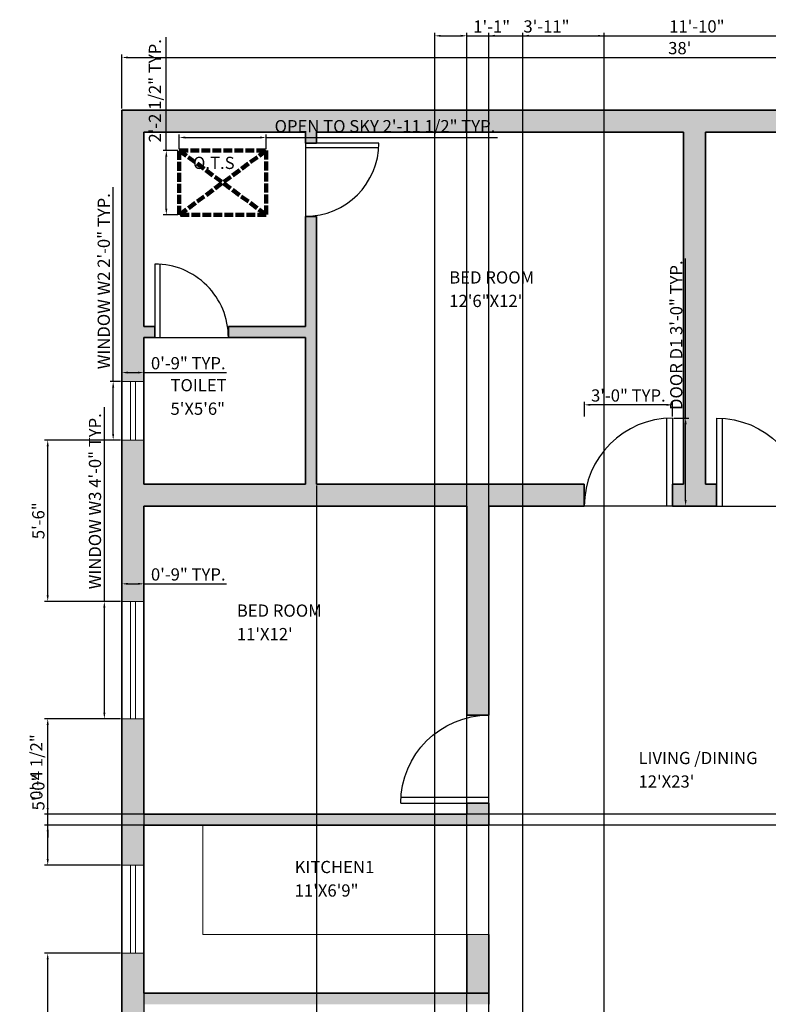
# Model space of a CAD drawing. Units: inches. Extents: x 2263 to 2802, y 2658 to 3310.
# Tile 2 of 3: x 2263 to 2569, y 2902 to 3305. Entities that reach past the tile are written whole.
import ezdxf

# ---------------------------------------------------------------- set-up
doc = ezdxf.new("R2010")
doc.units = ezdxf.units.IN
doc.header["$LTSCALE"] = 0.3
doc.linetypes.add('ACAD_ISO02W100', pattern=[15, 12, -3])
for name, color, linetype, lineweight in [('A-ANNO-DIMS', 2, 'Continuous', 18), ('A-AREA-IDEN', 7, 'Continuous', 18), ('A-DOOR', 3, 'Continuous', 25), ('A-FLOR-FIXT', 8, 'Continuous', 18), ('A-GLAZ', 4, 'Continuous', 18), ('A-ROOF-OVHD', 7, 'ACAD_ISO02W100', 100), ('A-WALL', 7, 'Continuous', 35)]:
    doc.layers.add(name, color=color, linetype=linetype, lineweight=lineweight)
doc.layers.add('A-WALL-PATT', color=18, linetype='Continuous', lineweight=13, true_color=0x000000)
doc.styles.get("Standard").update_dxf_attribs({"font": 'calibri.ttf', "height": 5})
doc.dimstyles.new('ISO-25', dxfattribs={"dimtxt": 5, "dimasz": 2.5, "dimexe": 1.25, "dimexo": 0.625, "dimtad": 1, "dimlunit": 3, "dimtxsty": 'Standard', "dimcen": 2.5, "dimadec": 0, "dimazin": 0, "dimtfac": 1, "dimtmove": 0, "dimatfit": 3, "dimfxl": 1, "dimarcsym": 0})

# ---------------------------------------------------------------- blocks, each defined once
blk = doc.blocks.new('*D1')
at = {"layer": 'A-ANNO-DIMS', "color": 0, "lineweight": -2, "transparency": 16777216}
for p, q in [((2304.41, 3268.9), (2304.41, 3291.01)), ((2760.41, 3268.9), (2760.41, 3291.01)), ((2306.91, 3289.76), (2757.91, 3289.76))]:
    blk.add_line(p, q, dxfattribs=at)
at = {"layer": 'A-ANNO-DIMS', "color": 0, "lineweight": -3, "transparency": 16777216}
for points in [[(2306.91, 3290.17), (2306.91, 3289.34), (2304.41, 3289.76)], [(2757.91, 3290.17), (2757.91, 3289.34), (2760.41, 3289.76)]]:
    blk.add_solid(points, dxfattribs=at)
at = {"layer": 'Defpoints', "color": 0, "lineweight": -3, "transparency": 16777216}
for p in [(2760.41, 3289.76), (2304.41, 3268.27), (2760.41, 3268.27)]:
    blk.add_point(p, dxfattribs=at)
at = {"layer": 'A-ANNO-DIMS', "color": 0, "transparency": 16777216, "insert": (2532.41, 3292.94), "char_height": 5, "attachment_point": 5}
blk.add_mtext("38'", dxfattribs=at)
blk = doc.blocks.new('DOOR-SWING-36')
for p, q in [((0, 0), (0, 36)), ((35.92, 2.4), (0, 2.4)), ((36, 0), (0, 0))]:
    blk.add_line(p, q)
blk.add_arc((0, 0), 36, 0, 90)
blk = doc.blocks.new('DOOR-SWING-30')
for p, q in [((30, 0), (0, 0)), ((0, 0), (0, -30)), ((29.93, -2), (0, -2))]:
    blk.add_line(p, q)
blk.add_arc((0, 0), 30, 270, 0)
blk = doc.blocks.new('WIN-24')
for p, q in [((0, 0), (0, -24)), ((9, 0), (0, 0)), ((3.5, 0), (3.5, -24)), ((5.5, 0), (5.5, -24)), ((9, -24), (9, 0)), ((0, -24), (9, -24))]:
    blk.add_line(p, q)
blk = doc.blocks.new('WIN-36')
for p, q in [((0, 36), (-9, 36)), ((-9, 36), (-9, 0)), ((-5.5, 0), (-5.5, 36)), ((-3.5, 0), (-3.5, 36)), ((0, 0), (0, 36)), ((-9, 0), (0, 0))]:
    blk.add_line(p, q)
blk = doc.blocks.new('WIN-48')
for p, q in [((0, 48), (-9, 48)), ((-9, 48), (-9, 0)), ((-5.5, 0), (-5.5, 48)), ((-3.5, 0), (-3.5, 48)), ((0, 0), (0, 48)), ((-9, 0), (0, 0))]:
    blk.add_line(p, q)
blk = doc.blocks.new('OPEN-TO-SKY')
for p, q in [((0, 0), (35.52, 0)), ((0, -26.28), (0, 0)), ((0, 0), (35.52, -26.28)), ((35.52, 0), (0, -26.28)), ((35.52, 0), (35.52, -26.28)), ((35.52, -26.28), (0, -26.28))]:
    blk.add_line(p, q)
blk = doc.blocks.new('*D9')
at = {"layer": 'A-ANNO-DIMS', "color": 0, "lineweight": -2, "transparency": 16777216}
for p, q in [((2534.81, 3142.27), (2534.81, 3207.54)), ((2530.03, 3142.27), (2536.06, 3142.27)), ((2534.81, 3108.77), (2534.81, 3139.77)), ((2530.03, 3106.27), (2536.06, 3106.27))]:
    blk.add_line(p, q, dxfattribs=at)
at = {"layer": 'A-ANNO-DIMS', "color": 0, "lineweight": -3, "transparency": 16777216}
for points in [[(2534.39, 3139.77), (2535.23, 3139.77), (2534.81, 3142.27)], [(2534.39, 3108.77), (2535.23, 3108.77), (2534.81, 3106.27)]]:
    blk.add_solid(points, dxfattribs=at)
at = {"layer": 'Defpoints', "color": 0, "lineweight": -3, "transparency": 16777216}
for p in [(2529.41, 3142.27), (2534.81, 3142.27), (2529.41, 3106.27)]:
    blk.add_point(p, dxfattribs=at)
at = {"layer": 'A-ANNO-DIMS', "color": 0, "transparency": 16777216, "insert": (2531.62, 3176.16), "char_height": 5, "attachment_point": 5, "rotation": 90}
blk.add_mtext('DOOR D1 3\'-0" TYP.', dxfattribs=at)
blk = doc.blocks.new('*D10')
at = {"layer": 'A-ANNO-DIMS', "color": 0, "lineweight": -2, "transparency": 16777216}
for p, q in [((2493.41, 3142.9), (2493.41, 3148.92)), ((2526.91, 3147.67), (2495.91, 3147.67)), ((2529.41, 3142.9), (2529.41, 3148.92))]:
    blk.add_line(p, q, dxfattribs=at)
at = {"layer": 'A-ANNO-DIMS', "color": 0, "lineweight": -3, "transparency": 16777216}
for points in [[(2495.91, 3148.09), (2495.91, 3147.26), (2493.41, 3147.67)], [(2526.91, 3148.09), (2526.91, 3147.26), (2529.41, 3147.67)]]:
    blk.add_solid(points, dxfattribs=at)
at = {"layer": 'Defpoints', "color": 0, "lineweight": -3, "transparency": 16777216}
for p in [(2493.41, 3147.67), (2493.41, 3142.27), (2529.41, 3142.27)]:
    blk.add_point(p, dxfattribs=at)
at = {"layer": 'A-ANNO-DIMS', "color": 0, "transparency": 16777216, "insert": (2511.41, 3150.86), "char_height": 5, "attachment_point": 5}
blk.add_mtext('3\'-0" TYP.', dxfattribs=at)
blk = doc.blocks.new('*D15')
at = {"layer": 'A-ANNO-DIMS', "color": 0, "lineweight": -2, "transparency": 16777216}
for p, q in [((2300.81, 3157.27), (2300.81, 3236.72)), ((2303.78, 3157.27), (2299.56, 3157.27)), ((2300.81, 3135.77), (2300.81, 3154.77)), ((2303.78, 3133.27), (2299.56, 3133.27))]:
    blk.add_line(p, q, dxfattribs=at)
at = {"layer": 'A-ANNO-DIMS', "color": 0, "lineweight": -3, "transparency": 16777216}
for points in [[(2300.39, 3154.77), (2301.23, 3154.77), (2300.81, 3157.27)], [(2300.39, 3135.77), (2301.23, 3135.77), (2300.81, 3133.27)]]:
    blk.add_solid(points, dxfattribs=at)
at = {"layer": 'Defpoints', "color": 0, "lineweight": -3, "transparency": 16777216}
for p in [(2300.81, 3157.27), (2304.41, 3157.27), (2304.41, 3133.27)]:
    blk.add_point(p, dxfattribs=at)
at = {"layer": 'A-ANNO-DIMS', "color": 0, "transparency": 16777216, "insert": (2297.62, 3198.25), "char_height": 5, "attachment_point": 5, "rotation": 90}
blk.add_mtext('WINDOW W2 2\'-0" TYP.', dxfattribs=at)
blk = doc.blocks.new('*D16')
at = {"layer": 'A-ANNO-DIMS', "color": 0, "lineweight": -2, "transparency": 16777216}
for p, q in [((2304.41, 3157.9), (2304.41, 3162.12)), ((2313.41, 3157.9), (2313.41, 3162.12)), ((2306.91, 3160.87), (2310.91, 3160.87)), ((2313.41, 3160.87), (2347.11, 3160.87))]:
    blk.add_line(p, q, dxfattribs=at)
at = {"layer": 'A-ANNO-DIMS', "color": 0, "lineweight": -3, "transparency": 16777216}
for points in [[(2306.91, 3161.29), (2306.91, 3160.46), (2304.41, 3160.87)], [(2310.91, 3161.29), (2310.91, 3160.46), (2313.41, 3160.87)]]:
    blk.add_solid(points, dxfattribs=at)
at = {"layer": 'Defpoints', "color": 0, "lineweight": -3, "transparency": 16777216}
for p in [(2313.41, 3160.87), (2304.41, 3157.27), (2313.41, 3157.27)]:
    blk.add_point(p, dxfattribs=at)
at = {"layer": 'A-ANNO-DIMS', "color": 0, "transparency": 16777216, "insert": (2331.51, 3164.06), "char_height": 5, "attachment_point": 5}
blk.add_mtext('0\'-9" TYP.', dxfattribs=at)
blk = doc.blocks.new('*D17')
at = {"layer": 'A-ANNO-DIMS', "color": 0, "lineweight": -2, "transparency": 16777216}
for p, q in [((2297.21, 3067.27), (2297.21, 3146.72)), ((2303.78, 3067.27), (2295.96, 3067.27)), ((2297.21, 3021.77), (2297.21, 3064.77)), ((2303.78, 3019.27), (2295.96, 3019.27))]:
    blk.add_line(p, q, dxfattribs=at)
at = {"layer": 'A-ANNO-DIMS', "color": 0, "lineweight": -3, "transparency": 16777216}
for points in [[(2296.79, 3064.77), (2297.63, 3064.77), (2297.21, 3067.27)], [(2296.79, 3021.77), (2297.63, 3021.77), (2297.21, 3019.27)]]:
    blk.add_solid(points, dxfattribs=at)
at = {"layer": 'Defpoints', "color": 0, "lineweight": -3, "transparency": 16777216}
for p in [(2297.21, 3067.27), (2304.41, 3067.27), (2304.41, 3019.27)]:
    blk.add_point(p, dxfattribs=at)
at = {"layer": 'A-ANNO-DIMS', "color": 0, "transparency": 16777216, "insert": (2294.02, 3108.25), "char_height": 5, "attachment_point": 5, "rotation": 90}
blk.add_mtext('WINDOW W3 4\'-0" TYP.', dxfattribs=at)
blk = doc.blocks.new('*D18')
at = {"layer": 'A-ANNO-DIMS', "color": 0, "lineweight": -2, "transparency": 16777216}
for p, q in [((2304.41, 3067.9), (2304.41, 3075.72)), ((2306.91, 3074.47), (2310.91, 3074.47)), ((2313.41, 3067.9), (2313.41, 3075.72)), ((2313.41, 3074.47), (2347.11, 3074.47))]:
    blk.add_line(p, q, dxfattribs=at)
at = {"layer": 'A-ANNO-DIMS', "color": 0, "lineweight": -3, "transparency": 16777216}
for points in [[(2306.91, 3074.89), (2306.91, 3074.06), (2304.41, 3074.47)], [(2310.91, 3074.89), (2310.91, 3074.06), (2313.41, 3074.47)]]:
    blk.add_solid(points, dxfattribs=at)
at = {"layer": 'Defpoints', "color": 0, "lineweight": -3, "transparency": 16777216}
for p in [(2313.41, 3074.47), (2304.41, 3067.27), (2313.41, 3067.27)]:
    blk.add_point(p, dxfattribs=at)
at = {"layer": 'A-ANNO-DIMS', "color": 0, "transparency": 16777216, "insert": (2331.51, 3077.66), "char_height": 5, "attachment_point": 5}
blk.add_mtext('0\'-9" TYP.', dxfattribs=at)
blk = doc.blocks.new('*D19')
at = {"layer": 'A-ANNO-DIMS', "color": 0, "lineweight": -2, "transparency": 16777216}
for p, q in [((2327.86, 3252.32), (2327.86, 3258.27)), ((2363.38, 3252.32), (2363.38, 3258.27)), ((2330.36, 3257.02), (2360.88, 3257.02)), ((2363.38, 3257.02), (2457.94, 3257.02))]:
    blk.add_line(p, q, dxfattribs=at)
at = {"layer": 'A-ANNO-DIMS', "color": 0, "lineweight": -3, "transparency": 16777216}
for points in [[(2330.36, 3257.44), (2330.36, 3256.6), (2327.86, 3257.02)], [(2360.88, 3257.44), (2360.88, 3256.6), (2363.38, 3257.02)]]:
    blk.add_solid(points, dxfattribs=at)
at = {"layer": 'Defpoints', "color": 0, "lineweight": -3, "transparency": 16777216}
for p in [(2363.38, 3257.02), (2327.86, 3251.69), (2363.38, 3251.69)]:
    blk.add_point(p, dxfattribs=at)
at = {"layer": 'A-ANNO-DIMS', "color": 0, "transparency": 16777216, "insert": (2411.91, 3261.01), "char_height": 5, "attachment_point": 5}
blk.add_mtext('OPEN TO SKY 2\'-11 1/2" TYP.', dxfattribs=at)
blk = doc.blocks.new('*D20')
at = {"layer": 'A-ANNO-DIMS', "color": 0, "lineweight": -2, "transparency": 16777216}
for p, q in [((2322.53, 3251.69), (2322.53, 3298.04)), ((2327.23, 3251.69), (2321.28, 3251.69)), ((2322.53, 3227.91), (2322.53, 3249.19)), ((2327.23, 3225.41), (2321.28, 3225.41))]:
    blk.add_line(p, q, dxfattribs=at)
at = {"layer": 'A-ANNO-DIMS', "color": 0, "lineweight": -3, "transparency": 16777216}
for points in [[(2322.12, 3249.19), (2322.95, 3249.19), (2322.53, 3251.69)], [(2322.12, 3227.91), (2322.95, 3227.91), (2322.53, 3225.41)]]:
    blk.add_solid(points, dxfattribs=at)
at = {"layer": 'Defpoints', "color": 0, "lineweight": -3, "transparency": 16777216}
for p in [(2322.53, 3251.69), (2327.86, 3251.69), (2327.86, 3225.41)]:
    blk.add_point(p, dxfattribs=at)
at = {"layer": 'A-ANNO-DIMS', "color": 0, "transparency": 16777216, "insert": (2318.54, 3276.12), "char_height": 5, "attachment_point": 5, "rotation": 90}
blk.add_mtext('2\'-2 1/2" TYP.', dxfattribs=at)
blk = doc.blocks.new('*D23')
at = {"layer": 'A-ANNO-DIMS', "color": 0, "lineweight": -2, "transparency": 16777216}
for p, q in [((2303.78, 2923.37), (2272.81, 2923.37)), ((2274.06, 2862.87), (2274.06, 2920.87)), ((2303.78, 2860.37), (2272.81, 2860.37))]:
    blk.add_line(p, q, dxfattribs=at)
at = {"layer": 'A-ANNO-DIMS', "color": 0, "lineweight": -3, "transparency": 16777216}
for points in [[(2273.64, 2920.87), (2274.48, 2920.87), (2274.06, 2923.37)], [(2273.64, 2862.87), (2274.48, 2862.87), (2274.06, 2860.37)]]:
    blk.add_solid(points, dxfattribs=at)
at = {"layer": 'Defpoints', "color": 0, "lineweight": -3, "transparency": 16777216}
for p in [(2274.06, 2923.37), (2304.41, 2923.37), (2304.41, 2860.37)]:
    blk.add_point(p, dxfattribs=at)
at = {"layer": 'A-ANNO-DIMS', "color": 0, "transparency": 16777216, "insert": (2270.87, 2891.87), "char_height": 5, "attachment_point": 5, "rotation": 90}
blk.add_mtext('5\'-3"', dxfattribs=at)
blk = doc.blocks.new('*D24')
at = {"layer": 'A-ANNO-DIMS', "color": 0, "lineweight": -2, "transparency": 16777216}
for p, q in [((2303.78, 3019.27), (2272.81, 3019.27)), ((2274.06, 2961.87), (2274.06, 3016.77)), ((2303.78, 2959.37), (2272.81, 2959.37))]:
    blk.add_line(p, q, dxfattribs=at)
at = {"layer": 'A-ANNO-DIMS', "color": 0, "lineweight": -3, "transparency": 16777216}
for points in [[(2273.64, 3016.77), (2274.48, 3016.77), (2274.06, 3019.27)], [(2273.64, 2961.87), (2274.48, 2961.87), (2274.06, 2959.37)]]:
    blk.add_solid(points, dxfattribs=at)
at = {"layer": 'Defpoints', "color": 0, "lineweight": -3, "transparency": 16777216}
for p in [(2274.06, 3019.27), (2304.41, 3019.27), (2304.41, 2959.37)]:
    blk.add_point(p, dxfattribs=at)
at = {"layer": 'A-ANNO-DIMS', "color": 0, "transparency": 16777216, "insert": (2270.87, 2989.32), "char_height": 5, "attachment_point": 5, "rotation": 90}
blk.add_mtext('5\'-0"', dxfattribs=at)
blk = doc.blocks.new('*D25')
at = {"layer": 'A-ANNO-DIMS', "color": 0, "lineweight": -2, "transparency": 16777216}
for p, q in [((2303.78, 3133.27), (2272.81, 3133.27)), ((2274.06, 3069.77), (2274.06, 3130.77)), ((2303.78, 3067.27), (2272.81, 3067.27))]:
    blk.add_line(p, q, dxfattribs=at)
at = {"layer": 'A-ANNO-DIMS', "color": 0, "lineweight": -3, "transparency": 16777216}
for points in [[(2273.64, 3130.77), (2274.48, 3130.77), (2274.06, 3133.27)], [(2273.64, 3069.77), (2274.48, 3069.77), (2274.06, 3067.27)]]:
    blk.add_solid(points, dxfattribs=at)
at = {"layer": 'Defpoints', "color": 0, "lineweight": -3, "transparency": 16777216}
for p in [(2274.06, 3133.27), (2304.41, 3133.27), (2304.41, 3067.27)]:
    blk.add_point(p, dxfattribs=at)
at = {"layer": 'A-ANNO-DIMS', "color": 0, "transparency": 16777216, "insert": (2270.87, 3100.27), "char_height": 5, "attachment_point": 5, "rotation": 90}
blk.add_mtext('5\'-6"', dxfattribs=at)
blk = doc.blocks.new('*D29')
at = {"layer": 'A-ANNO-DIMS', "color": 0, "lineweight": -2, "transparency": 16777216}
for p, q in [((2454.41, 2770.9), (2454.41, 3299.87)), ((2456.91, 3298.62), (2498.96, 3298.62)), ((2501.46, 2770.9), (2501.46, 3299.87))]:
    blk.add_line(p, q, dxfattribs=at)
at = {"layer": 'A-ANNO-DIMS', "color": 0, "lineweight": -3, "transparency": 16777216}
for points in [[(2456.91, 3299.04), (2456.91, 3298.21), (2454.41, 3298.62)], [(2498.96, 3299.04), (2498.96, 3298.21), (2501.46, 3298.62)]]:
    blk.add_solid(points, dxfattribs=at)
at = {"layer": 'Defpoints', "color": 0, "lineweight": -3, "transparency": 16777216}
for p in [(2501.46, 3298.62), (2454.41, 2770.27), (2501.46, 2770.27)]:
    blk.add_point(p, dxfattribs=at)
at = {"layer": 'A-ANNO-DIMS', "color": 0, "transparency": 16777216, "insert": (2477.93, 3301.81), "char_height": 5, "attachment_point": 5}
blk.add_mtext('3\'-11"', dxfattribs=at)
blk = doc.blocks.new('*D31')
at = {"layer": 'A-ANNO-DIMS', "color": 0, "lineweight": -2, "transparency": 16777216}
for p, q in [((2432.25, 2770.9), (2432.25, 3299.87)), ((2434.75, 3298.62), (2442.91, 3298.62)), ((2445.41, 2770.9), (2445.41, 3299.87)), ((2445.41, 3298.62), (2463.19, 3298.62))]:
    blk.add_line(p, q, dxfattribs=at)
at = {"layer": 'A-ANNO-DIMS', "color": 0, "lineweight": -3, "transparency": 16777216}
for points in [[(2434.75, 3299.04), (2434.75, 3298.21), (2432.25, 3298.62)], [(2442.91, 3299.04), (2442.91, 3298.21), (2445.41, 3298.62)]]:
    blk.add_solid(points, dxfattribs=at)
at = {"layer": 'Defpoints', "color": 0, "lineweight": -3, "transparency": 16777216}
for p in [(2445.41, 3298.62), (2432.25, 2770.27), (2445.41, 2770.27)]:
    blk.add_point(p, dxfattribs=at)
at = {"layer": 'A-ANNO-DIMS', "color": 0, "transparency": 16777216, "insert": (2455.55, 3301.75), "char_height": 5, "attachment_point": 5}
blk.add_mtext('1\'-1"', dxfattribs=at)
blk = doc.blocks.new('*D35')
at = {"layer": 'A-ANNO-DIMS', "color": 0, "lineweight": -2, "transparency": 16777216}
for p, q in [((2274.06, 2982.77), (2274.06, 3013.75)), ((2618.78, 2980.27), (2272.81, 2980.27)), ((2274.06, 2975.77), (2274.06, 2980.27)), ((2609.78, 2975.77), (2272.81, 2975.77)), ((2274.06, 2973.27), (2274.06, 2970.77))]:
    blk.add_line(p, q, dxfattribs=at)
at = {"layer": 'A-ANNO-DIMS', "color": 0, "lineweight": -3, "transparency": 16777216}
for points in [[(2273.64, 2982.77), (2274.48, 2982.77), (2274.06, 2980.27)], [(2273.64, 2973.27), (2274.48, 2973.27), (2274.06, 2975.77)]]:
    blk.add_solid(points, dxfattribs=at)
at = {"layer": 'Defpoints', "color": 0, "lineweight": -3, "transparency": 16777216}
for p in [(2274.06, 2980.27), (2619.41, 2980.27), (2610.41, 2975.77)]:
    blk.add_point(p, dxfattribs=at)
at = {"layer": 'A-ANNO-DIMS', "color": 0, "transparency": 16777216, "insert": (2270.07, 2999.51), "char_height": 5, "attachment_point": 5, "rotation": 90}
blk.add_mtext('0\'-4 1/2"', dxfattribs=at)
blk = doc.blocks.new('*D42')
at = {"layer": 'A-ANNO-DIMS', "color": 0, "lineweight": -2, "transparency": 16777216}
for p, q in [((2468.29, 2867.1), (2468.29, 3299.87)), ((2470.79, 3298.62), (2608, 3298.62)), ((2610.5, 2867.1), (2610.5, 3299.87))]:
    blk.add_line(p, q, dxfattribs=at)
at = {"layer": 'A-ANNO-DIMS', "color": 0, "lineweight": -3, "transparency": 16777216}
for points in [[(2470.79, 3299.04), (2470.79, 3298.21), (2468.29, 3298.62)], [(2608, 3299.04), (2608, 3298.21), (2610.5, 3298.62)]]:
    blk.add_solid(points, dxfattribs=at)
at = {"layer": 'Defpoints', "color": 0, "lineweight": -3, "transparency": 16777216}
for p in [(2610.5, 3298.62), (2468.29, 2866.48), (2610.5, 2866.48)]:
    blk.add_point(p, dxfattribs=at)
at = {"layer": 'A-ANNO-DIMS', "color": 0, "transparency": 16777216, "insert": (2539.4, 3301.81), "char_height": 5, "attachment_point": 5}
blk.add_mtext('11\'-10"', dxfattribs=at)
blk = doc.blocks.new('*D43')
at = {"layer": 'A-ANNO-DIMS', "color": 0, "lineweight": -2, "transparency": 16777216}
for p, q in [((2383.91, 3114.65), (2383.91, 2660.67)), ((2313.41, 3105.65), (2313.41, 2660.67)), ((2315.91, 2661.92), (2381.41, 2661.92))]:
    blk.add_line(p, q, dxfattribs=at)
at = {"layer": 'A-ANNO-DIMS', "color": 0, "lineweight": -3, "transparency": 16777216}
for points in [[(2315.91, 2662.34), (2315.91, 2661.51), (2313.41, 2661.92)], [(2381.41, 2662.34), (2381.41, 2661.51), (2383.91, 2661.92)]]:
    blk.add_solid(points, dxfattribs=at)
at = {"layer": 'Defpoints', "color": 0, "lineweight": -3, "transparency": 16777216}
for p in [(2383.91, 3115.27), (2313.41, 3106.27), (2383.91, 2661.92)]:
    blk.add_point(p, dxfattribs=at)
at = {"layer": 'A-ANNO-DIMS', "color": 0, "transparency": 16777216, "insert": (2348.66, 2665.91), "char_height": 5, "attachment_point": 5}
blk.add_mtext('5\'-10 1/2"', dxfattribs=at)

msp = doc.modelspace()

# ---------------------------------------------------------------- hatches: boundary and pattern name
at = {"layer": 'A-WALL-PATT'}
h = msp.add_hatch(color=256, dxfattribs=at)
h.dxf.hatch_style = 1
h.paths.add_polyline_path([(2454.409, 2984.773), (2445.409, 2984.773), (2445.409, 2980.273), (2313.409, 2980.273), (2313.409, 3019.273), (2304.409, 3019.273), (2304.409, 2959.375), (2313.409, 2959.375), (2313.409, 2975.773), (2454.409, 2975.773)], flags=17)
h.paths.add_polyline_path([(2313.409, 2902.477), (2454.409, 2902.477), (2454.409, 2906.977), (2313.409, 2906.977), (2313.409, 2923.375), (2304.409, 2923.375), (2304.409, 2860.375), (2313.409, 2860.375)], flags=17)
h.paths.add_polyline_path([(2313.409, 2812.375), (2304.409, 2812.375), (2304.409, 2692.273), (2334.409, 2692.273), (2334.409, 2701.273), (2313.409, 2701.273), (2313.409, 2761.273), (2379.409, 2761.273), (2379.409, 2735.773), (2383.909, 2735.773), (2383.909, 2761.273), (2396.251, 2761.273), (2396.251, 2770.273), (2313.409, 2770.273)], flags=17)
h.paths.add_polyline_path([(2760.409, 3268.273), (2304.409, 3268.273), (2304.409, 3157.273), (2313.409, 3157.273), (2313.409, 3175.273), (2317.909, 3175.273), (2317.909, 3179.773), (2313.409, 3179.773), (2313.409, 3259.273), (2379.409, 3259.273), (2379.409, 3254.773), (2383.909, 3254.773), (2383.909, 3259.273), (2533.909, 3259.273), (2533.909, 3115.273), (2529.409, 3115.273), (2529.409, 3106.273), (2547.409, 3106.273), (2547.409, 3115.273), (2542.909, 3115.273), (2542.909, 3259.273), (2692.909, 3259.273), (2692.909, 3254.773), (2697.409, 3254.773), (2697.409, 3259.273), (2751.409, 3259.273), (2751.409, 3179.773), (2746.909, 3179.773), (2746.909, 3175.273), (2751.409, 3175.273), (2751.409, 3115.273), (2697.409, 3115.273), (2697.409, 3175.273), (2716.909, 3175.273), (2716.909, 3179.773), (2697.409, 3179.773), (2697.409, 3224.773), (2692.909, 3224.773), (2692.909, 3115.273), (2583.409, 3115.273), (2583.409, 3106.273), (2610.409, 3106.273), (2610.409, 3090.217), (2619.409, 3090.217), (2619.409, 3106.273), (2751.409, 3106.273), (2751.409, 2980.273), (2619.409, 2980.273), (2619.409, 2984.773), (2610.409, 2984.773), (2610.409, 2975.773), (2751.409, 2975.773), (2751.409, 2906.977), (2634.409, 2906.977), (2634.409, 2902.477), (2670.409, 2902.477), (2751.409, 2902.477), (2751.409, 2701.273), (2383.909, 2701.273), (2383.909, 2705.773), (2379.409, 2705.773), (2379.409, 2701.273), (2358.409, 2701.273), (2358.409, 2692.273), (2760.409, 2692.273)])
h.paths.add_polyline_path([(2501.459, 2770.273), (2454.409, 2770.273), (2454.409, 2857.477), (2468.293, 2857.477), (2468.293, 2866.477), (2445.409, 2866.477), (2445.409, 2770.273), (2432.251, 2770.273), (2432.251, 2761.273), (2501.459, 2761.273)], flags=17)
h.paths.add_polyline_path([(2593.909, 2770.273), (2573.459, 2770.273), (2573.459, 2761.273), (2593.909, 2761.273)], flags=17)
h.paths.add_polyline_path([(2643.409, 2866.477), (2610.501, 2866.477), (2610.501, 2857.477), (2634.409, 2857.477), (2634.409, 2770.273), (2629.909, 2770.273), (2629.909, 2761.273), (2643.409, 2761.273)], flags=17)
h.paths.add_polyline_path([(2643.409, 2930.977), (2634.409, 2930.977), (2634.409, 2906.977), (2643.409, 2906.977)], flags=17)
h.paths.add_polyline_path([(2454.409, 2930.977), (2445.409, 2930.977), (2445.409, 2906.977), (2454.409, 2906.977)], flags=17)
h.paths.add_polyline_path([(2454.409, 3106.273), (2493.409, 3106.273), (2493.409, 3115.273), (2383.909, 3115.273), (2383.909, 3224.773), (2379.409, 3224.773), (2379.409, 3179.773), (2347.909, 3179.773), (2347.909, 3175.273), (2379.409, 3175.273), (2379.409, 3115.273), (2313.409, 3115.273), (2313.409, 3133.273), (2304.409, 3133.273), (2304.409, 3067.273), (2313.409, 3067.273), (2313.409, 3106.273), (2445.409, 3106.273), (2445.409, 3020.773), (2454.409, 3020.773)], flags=17)
h.paths.add_polyline_path([(2619.409, 3054.217), (2610.409, 3054.217), (2610.409, 3020.773), (2619.409, 3020.773)], flags=17)

# ---------------------------------------------------------------- linework, layer by layer
at = {"layer": 'A-FLOR-FIXT'}
for q in [(2337.409, 2975.773), (2454.409, 2930.977)]:
    msp.add_line((2337.409, 2930.977), q, dxfattribs=at)
at = {"layer": 'A-WALL'}
for p, q in [((2304.409, 3268.273), (2760.409, 3268.273)), ((2304.409, 2692.273), (2304.409, 3268.273)), ((2313.409, 3259.273), (2379.409, 3259.273)), ((2313.409, 3179.773), (2313.409, 3259.273)), ((2379.409, 3254.773), (2379.409, 3259.273)), ((2383.909, 3259.273), (2533.909, 3259.273)), ((2383.909, 3254.773), (2383.909, 3259.273)), ((2533.909, 3115.273), (2533.909, 3259.273)), ((2542.909, 3115.273), (2542.909, 3259.273)), ((2542.909, 3259.273), (2692.909, 3259.273)), ((2379.409, 3254.773), (2383.909, 3254.773)), ((2379.409, 3179.773), (2379.409, 3224.773)), ((2379.409, 3224.773), (2383.909, 3224.773)), ((2383.909, 3115.273), (2383.909, 3224.773)), ((2313.409, 3179.773), (2317.909, 3179.773)), ((2317.909, 3179.773), (2317.909, 3175.273)), ((2347.909, 3179.773), (2347.909, 3175.273)), ((2347.909, 3179.773), (2379.409, 3179.773)), ((2313.409, 3175.273), (2317.909, 3175.273)), ((2313.409, 3115.273), (2313.409, 3175.273)), ((2347.909, 3175.273), (2379.409, 3175.273)), ((2379.409, 3115.273), (2379.409, 3175.273)), ((2313.409, 3115.273), (2379.409, 3115.273)), ((2383.909, 3115.273), (2493.409, 3115.273)), ((2493.409, 3115.273), (2493.409, 3106.273)), ((2529.409, 3115.273), (2529.409, 3106.273)), ((2529.409, 3115.273), (2533.909, 3115.273)), ((2542.909, 3115.273), (2547.409, 3115.273)), ((2547.409, 3115.273), (2547.409, 3106.273)), ((2313.409, 3106.273), (2445.409, 3106.273)), ((2313.409, 2980.273), (2313.409, 3106.273)), ((2445.409, 3020.773), (2445.409, 3106.273)), ((2454.409, 3106.273), (2454.409, 3020.773)), ((2454.409, 3106.273), (2493.409, 3106.273)), ((2454.409, 3020.773), (2454.409, 3106.273)), ((2529.409, 3106.273), (2547.409, 3106.273)), ((2445.409, 3020.773), (2454.409, 3020.773)), ((2445.409, 2980.273), (2445.409, 2984.773)), ((2445.409, 2984.773), (2454.409, 2984.773)), ((2454.409, 2975.773), (2454.409, 2984.773)), ((2454.409, 2984.773), (2454.409, 2980.273)), ((2313.409, 2980.273), (2445.409, 2980.273)), ((2313.409, 2975.773), (2454.409, 2975.773)), ((2313.409, 2906.977), (2313.409, 2975.773)), ((2445.409, 2930.977), (2445.409, 2906.977)), ((2454.409, 2930.977), (2454.409, 2906.977)), ((2313.409, 2906.977), (2454.409, 2906.977)), ((2454.409, 2906.977), (2454.409, 2902.477))]:
    msp.add_line(p, q, dxfattribs=at)

# ---------------------------------------------------------------- block references
at = {"layer": 'A-DOOR'}
msp.add_blockref('DOOR-SWING-30', (2379.409, 3254.773), dxfattribs=at)
for name, p, rotation in [('DOOR-SWING-30', (2317.909, 3175.273), 90.00000000000561), ('DOOR-SWING-36', (2529.409, 3106.273), 90.00000000000026)]:
    msp.add_blockref(name, p, dxfattribs=dict(at, rotation=rotation))
at = {"layer": 'A-DOOR', "extrusion": (0, 0, -1), "zscale": -1, "rotation": 89.99999999999883}
msp.add_blockref('DOOR-SWING-36', (-2547.409, 3106.273), dxfattribs=at)
at = {"layer": 'A-DOOR', "extrusion": (0, 0, -1), "zscale": -1}
msp.add_blockref('DOOR-SWING-36', (-2454.409, 2984.773), dxfattribs=at)
at = {"layer": 'A-GLAZ'}
for name, p in [('WIN-24', (2304.409, 3157.273)), ('WIN-48', (2313.409, 3019.273))]:
    msp.add_blockref(name, p, dxfattribs=at)
at = {"layer": 'A-GLAZ', "rotation": 180}
msp.add_blockref('WIN-36', (2304.409, 2959.375), dxfattribs=at)
at = {"layer": 'A-ROOF-OVHD'}
msp.add_blockref('OPEN-TO-SKY', (2327.86, 3251.693), dxfattribs=at)

# ---------------------------------------------------------------- texts
at = {"layer": 'A-AREA-IDEN'}
for s, p in [('O.T.S', (2333.452, 3244.141)), ('BED ROOM', (2438.196, 3197.299)), ('12\'6"X12\'', (2438.196, 3187.684)), ('TOILET', (2324.246, 3153.209)), ('5\'X5\'6"', (2324.246, 3143.594)), ('BED ROOM', (2351.358, 3061.015)), ("11'X12'", (2351.358, 3051.4)), ('LIVING /DINING', (2515.546, 3000.718)), ("12'X23'", (2515.546, 2991.103)), ('KITCHEN1', (2375.012, 2956.143)), ('11\'X6\'9"', (2375.012, 2946.528))]:
    msp.add_text(s, height=5, dxfattribs=at).set_placement(p)

# ---------------------------------------------------------------- dimensions: what is measured, and where the dimension line sits
at = {"layer": 'A-ANNO-DIMS'}
for base, p1, p2, override, picture, middle in [((2445.409, 3298.623), (2432.251, 2770.273), (2445.409, 2770.273), {"dimdec": 1, "dimlfac": 1, "dimrnd": 0, "dimzin": 1, "dimdsep": 46, "dimlunit": 4, "dimfrac": 2}, '*D31', (2455.548, 3301.753)), ((2501.459, 3298.6226), (2454.4094, 2770.2726), (2501.459, 2770.2726), {"dimdec": 1, "dimlfac": 1, "dimrnd": 0, "dimzin": 1, "dimdsep": 46, "dimlunit": 4, "dimfrac": 2}, '*D29', (2477.9342, 3301.8092)), ((2610.501, 3298.623), (2468.293, 2866.477), (2610.501, 2866.477), {"dimdec": 1, "dimlfac": 1, "dimrnd": 0, "dimzin": 1, "dimdsep": 46, "dimlunit": 4, "dimfrac": 2}, '*D42', (2539.397, 3301.809)), ((2760.409, 3289.757), (2304.409, 3268.273), (2760.409, 3268.273), {"dimclrd": 0, "dimclre": 0, "dimclrt": 0}, '*D1', (2532.409, 3292.944)), ((2383.909, 2661.923), (2313.409, 3106.273), (2383.909, 3115.273), {"dimdec": 1, "dimlfac": 1, "dimrnd": 0, "dimzin": 1, "dimdsep": 46, "dimlunit": 4, "dimfrac": 2}, '*D43', (2348.659, 2665.915))]:
    dim = msp.add_linear_dim(base=base, p1=p1, p2=p2, dimstyle='ISO-25', override=override, dxfattribs=at)
    dim.commit()
    dim.dimension.update_dxf_attribs({"geometry": picture, "text_midpoint": middle})
for base, p1, p2, angle, text, picture, middle in [((2322.532, 3251.693), (2327.86, 3225.411), (2327.86, 3251.693), 90, '<> TYP.', '*D20', (2318.54, 3276.116)), ((2300.809, 3157.273), (2304.409, 3133.273), (2304.409, 3157.273), 90, 'WINDOW W2 <> TYP.', '*D15', (2297.623, 3198.248)), ((2534.809, 3142.273), (2529.409, 3106.273), (2529.409, 3142.273), 90, 'DOOR D1 <> TYP.', '*D9', (2531.623, 3176.157)), ((2493.409, 3147.673), (2529.409, 3142.273), (2493.409, 3142.273), 180, '<> TYP.', '*D10', (2511.409, 3150.859)), ((2297.209, 3067.273), (2304.409, 3019.273), (2304.409, 3067.273), 90, 'WINDOW W3 <> TYP.', '*D17', (2294.023, 3108.248))]:
    dim = msp.add_linear_dim(base=base, p1=p1, p2=p2, angle=angle, text=text, dimstyle='ISO-25', override={"dimdec": 1, "dimlfac": 1, "dimrnd": 0, "dimzin": 1, "dimdsep": 46, "dimlunit": 4, "dimfrac": 2}, dxfattribs=at)
    dim.commit()
    dim.dimension.update_dxf_attribs({"geometry": picture, "text_midpoint": middle})
for base, p1, p2, text, picture, middle in [((2363.378, 3257.021), (2327.86, 3251.693), (2363.378, 3251.693), 'OPEN TO SKY <> TYP.', '*D19', (2411.907, 3261.013)), ((2313.409, 3160.873), (2304.409, 3157.273), (2313.409, 3157.273), '<> TYP.', '*D16', (2331.509, 3164.059)), ((2313.409, 3074.473), (2304.409, 3067.273), (2313.409, 3067.273), '<> TYP.', '*D18', (2331.509, 3077.659))]:
    dim = msp.add_linear_dim(base=base, p1=p1, p2=p2, text=text, dimstyle='ISO-25', override={"dimdec": 1, "dimlfac": 1, "dimrnd": 0, "dimzin": 1, "dimdsep": 46, "dimlunit": 4, "dimfrac": 2}, dxfattribs=at)
    dim.commit()
    dim.dimension.update_dxf_attribs({"geometry": picture, "text_midpoint": middle})
for base, p1, p2, picture, middle in [((2274.059, 3133.273), (2304.409, 3067.273), (2304.409, 3133.273), '*D25', (2270.875, 3100.273)), ((2274.059, 3019.273), (2304.409, 2959.375), (2304.409, 3019.273), '*D24', (2270.873, 2989.324)), ((2274.059, 2980.273), (2610.409, 2975.773), (2619.409, 2980.273), '*D35', (2270.067, 2999.511)), ((2274.059, 2923.375), (2304.409, 2860.375), (2304.409, 2923.375), '*D23', (2270.873, 2891.875))]:
    dim = msp.add_linear_dim(base=base, p1=p1, p2=p2, angle=90, dimstyle='ISO-25', override={"dimdec": 1, "dimlfac": 1, "dimrnd": 0, "dimzin": 1, "dimdsep": 46, "dimlunit": 4, "dimfrac": 2}, dxfattribs=at)
    dim.commit()
    dim.dimension.update_dxf_attribs({"geometry": picture, "text_midpoint": middle})

doc.saveas('drawing.dxf')
